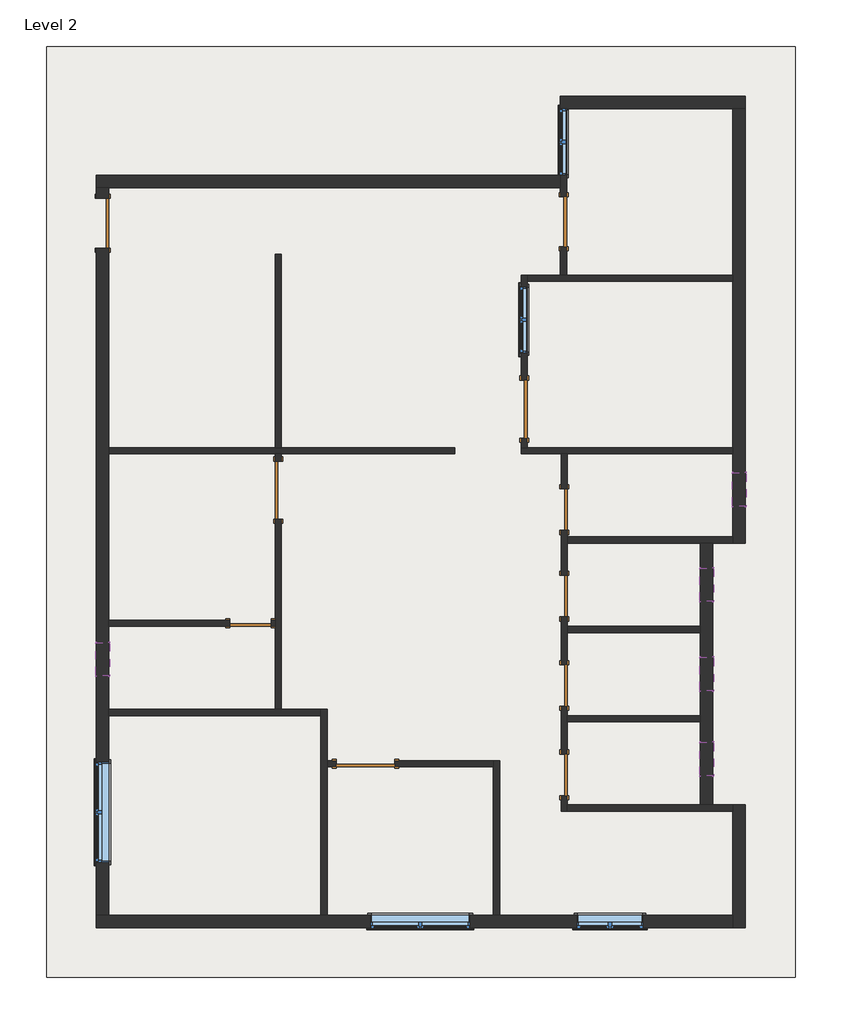
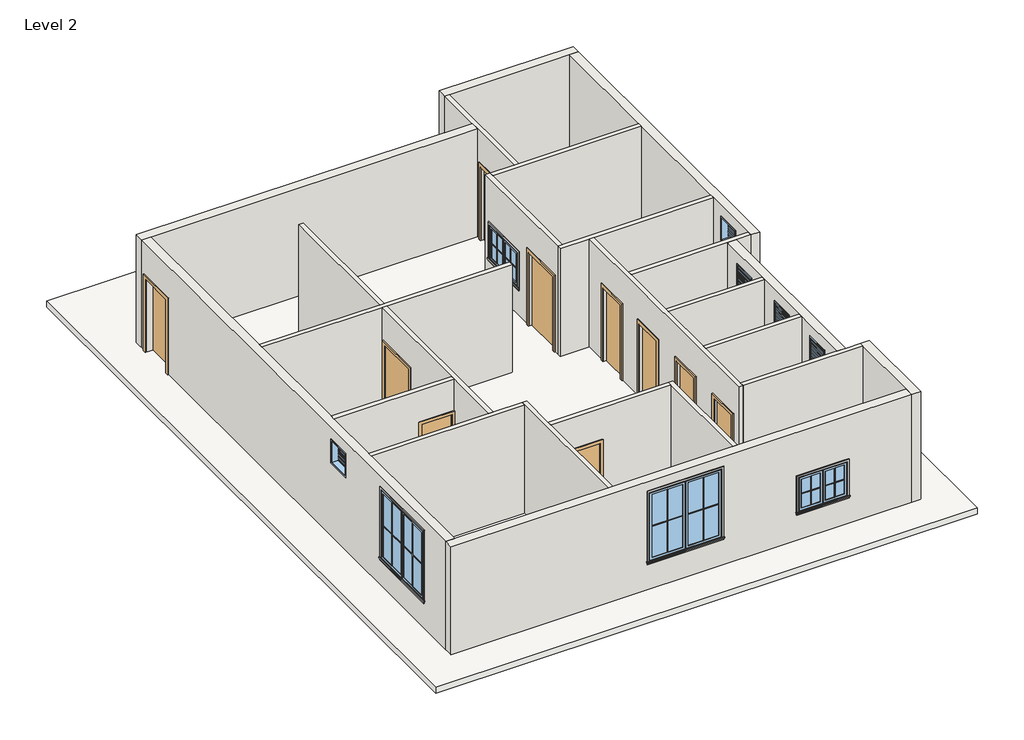
# One storey, incomplete: 23 walls, 20 proxies, 10 doors, 10 windows, 1 roof.
"""IFC4 building model written with IfcOpenShell, lengths in millimetres."""

from ifc_helpers import new_model, si_unit, frame, origin, place, context, project, spatial, polyline, outline, extrude, faceted_brep, transform, mapped, element, save
from components import muntin_pattern_2x2_muntin_pattern_2x2_0a037076, muntin_pattern_2x2_muntin_pattern_2x2_e6f69628, muntin_pattern_2x2_muntin_pattern_2x2_2357e71d, muntin_pattern_2x2_muntin_pattern_2x2_302d8f29, trim_window_exterior_flat_with_sill_b601e94a, trim_window_exterior_flat_with_sill_c4e67c73, trim_window_interior_flat_picture_frame_bfefb25c, trim_window_interior_flat_picture_frame_cf1733af, door_78caadf7, door_214872d5, single_flush_door_3_305aa2a5, single_flush_door_3_a90ba1ad, door_4c162e62, window_casement_double_win_4_c19c33cb, window_casement_double_win_4_2967420f, window_casement_double_win_6_ce442eab, window_f2d8fef0

model = new_model("IFC4")

# Units and contexts
model_context = context("Model", 3, world=origin())
ifc_project = project(units=[si_unit("LENGTHUNIT", "METRE", prefix="MILLI")], contexts=[model_context])

# Site, building, storey
site = spatial("IfcSite", under=ifc_project)
building = spatial("IfcBuilding", under=site)
storey = spatial("IfcBuildingStorey", under=building, Name="Level 2", Elevation=3048.0)

# Proxies
placement = place(None, origin())
muntin_pattern_2x2_muntin_pattern_2x2_shape = muntin_pattern_2x2_muntin_pattern_2x2_0a037076(model_context)
element("IfcBuildingElementProxy", 1, Name="Muntin Pattern_2x2 : Muntin Pattern_2x2", ObjectType="Muntin Pattern_2x2 : Muntin Pattern_2x2", at=placement, inside=storey, context=model_context, shape_type="MappedRepresentation", body=[
    mapped(muntin_pattern_2x2_muntin_pattern_2x2_shape, transform((-7058.058853, -4848.517381, 4032.25), x_axis=(0.0, 1.0, 0.0), y_axis=(-1.0, 0.0, 0.0), z_axis=(0.0, 0.0, 1.0))),
])
element("IfcBuildingElementProxy", 2, Name="Muntin Pattern_2x2 : Muntin Pattern_2x2", ObjectType="Muntin Pattern_2x2 : Muntin Pattern_2x2", at=placement, inside=storey, context=model_context, shape_type="MappedRepresentation", body=[
    mapped(muntin_pattern_2x2_muntin_pattern_2x2_shape, transform((-674.721353, -6497.929881, 4032.25), x_axis=(-1.0, 0.0, 0.0), y_axis=(0.0, -1.0, 0.0), z_axis=(0.0, 0.0, 1.0))),
])
muntin_pattern_2x2_muntin_pattern_2x2_2_shape = muntin_pattern_2x2_muntin_pattern_2x2_e6f69628(model_context)
element("IfcBuildingElementProxy", 3, Name="Muntin Pattern_2x2 : Muntin Pattern_2x2", ObjectType="Muntin Pattern_2x2 : Muntin Pattern_2x2", at=placement, inside=storey, context=model_context, shape_type="MappedRepresentation", body=[
    mapped(muntin_pattern_2x2_muntin_pattern_2x2_2_shape, transform((-7058.058853, -3937.292381, 4032.25), x_axis=(0.0, -1.0, 0.0), y_axis=(1.0, 0.0, 0.0), z_axis=(0.0, 0.0, 1.0))),
])
element("IfcBuildingElementProxy", 4, Name="Muntin Pattern_2x2 : Muntin Pattern_2x2", ObjectType="Muntin Pattern_2x2 : Muntin Pattern_2x2", at=placement, inside=storey, context=model_context, shape_type="MappedRepresentation", body=[
    mapped(muntin_pattern_2x2_muntin_pattern_2x2_2_shape, transform((-1585.946353, -6497.929881, 4032.25), x_axis=(1.0, 0.0, 0.0), y_axis=(0.0, 1.0, 0.0), z_axis=(0.0, 0.0, 1.0))),
])
muntin_pattern_2x2_muntin_pattern_2x2_3_shape = muntin_pattern_2x2_muntin_pattern_2x2_2357e71d(model_context)
element("IfcBuildingElementProxy", 5, Name="Muntin Pattern_2x2 : Muntin Pattern_2x2", ObjectType="Muntin Pattern_2x2 : Muntin Pattern_2x2", at=placement, inside=storey, context=model_context, shape_type="MappedRepresentation", body=[
    mapped(muntin_pattern_2x2_muntin_pattern_2x2_3_shape, transform((2652.678647, -6497.929881, 4032.25), x_axis=(-1.0, 0.0, 0.0), y_axis=(0.0, -1.0, 0.0), z_axis=(0.0, 0.0, 1.0))),
])
element("IfcBuildingElementProxy", 6, Name="Muntin Pattern_2x2 : Muntin Pattern_2x2", ObjectType="Muntin Pattern_2x2 : Muntin Pattern_2x2", at=placement, inside=storey, context=model_context, shape_type="MappedRepresentation", body=[
    mapped(muntin_pattern_2x2_muntin_pattern_2x2_3_shape, transform((727.041147, 4333.582619, 4032.25), x_axis=(0.0, 1.0, 0.0), y_axis=(-1.0, 0.0, 0.0), z_axis=(0.0, 0.0, 1.0))),
])
element("IfcBuildingElementProxy", 7, Name="Muntin Pattern_2x2 : Muntin Pattern_2x2", ObjectType="Muntin Pattern_2x2 : Muntin Pattern_2x2", at=placement, inside=storey, context=model_context, shape_type="MappedRepresentation", body=[
    mapped(muntin_pattern_2x2_muntin_pattern_2x2_3_shape, transform((1450.941147, 7591.132619, 4032.25), x_axis=(0.0, 1.0, 0.0), y_axis=(-1.0, 0.0, 0.0), z_axis=(0.0, 0.0, 1.0))),
])
muntin_pattern_2x2_muntin_pattern_2x2_4_shape = muntin_pattern_2x2_muntin_pattern_2x2_302d8f29(model_context)
element("IfcBuildingElementProxy", 8, Name="Muntin Pattern_2x2 : Muntin Pattern_2x2", ObjectType="Muntin Pattern_2x2 : Muntin Pattern_2x2", at=placement, inside=storey, context=model_context, shape_type="MappedRepresentation", body=[
    mapped(muntin_pattern_2x2_muntin_pattern_2x2_4_shape, transform((2046.253647, -6497.929881, 4032.25), x_axis=(1.0, 0.0, 0.0), y_axis=(0.0, 1.0, 0.0), z_axis=(0.0, 0.0, 1.0))),
])
element("IfcBuildingElementProxy", 9, Name="Muntin Pattern_2x2 : Muntin Pattern_2x2", ObjectType="Muntin Pattern_2x2 : Muntin Pattern_2x2", at=placement, inside=storey, context=model_context, shape_type="MappedRepresentation", body=[
    mapped(muntin_pattern_2x2_muntin_pattern_2x2_4_shape, transform((727.041147, 4940.007619, 4032.25), x_axis=(0.0, -1.0, 0.0), y_axis=(1.0, 0.0, 0.0), z_axis=(0.0, 0.0, 1.0))),
])
element("IfcBuildingElementProxy", 10, Name="Muntin Pattern_2x2 : Muntin Pattern_2x2", ObjectType="Muntin Pattern_2x2 : Muntin Pattern_2x2", at=placement, inside=storey, context=model_context, shape_type="MappedRepresentation", body=[
    mapped(muntin_pattern_2x2_muntin_pattern_2x2_4_shape, transform((1450.941147, 8197.557619, 4032.25), x_axis=(0.0, -1.0, 0.0), y_axis=(1.0, 0.0, 0.0), z_axis=(0.0, 0.0, 1.0))),
])
trim_window_exterior_flat_with_sill_shape = trim_window_exterior_flat_with_sill_b601e94a(model_context)
element("IfcBuildingElementProxy", 11, Name="Trim-Window-Exterior-Flat : with Sill", ObjectType="Trim-Window-Exterior-Flat : with Sill", at=placement, inside=storey, context=model_context, shape_type="MappedRepresentation", body=[
    mapped(trim_window_exterior_flat_with_sill_shape, transform((-7067.583853, -4392.904881, 5791.2), x_axis=(0.0, -1.0, 0.0), y_axis=(0.0, 0.0, 1.0), z_axis=(-1.0, 0.0, 0.0))),
])
element("IfcBuildingElementProxy", 12, Name="Trim-Window-Exterior-Flat : with Sill", ObjectType="Trim-Window-Exterior-Flat : with Sill", at=placement, inside=storey, context=model_context, shape_type="MappedRepresentation", body=[
    mapped(trim_window_exterior_flat_with_sill_shape, transform((-1130.333853, -6507.454881, 5791.2), x_axis=(1.0, 0.0, 0.0), y_axis=(0.0, 0.0, 1.0), z_axis=(0.0, -1.0, 0.0))),
])
trim_window_exterior_flat_with_sill_2_shape = trim_window_exterior_flat_with_sill_c4e67c73(model_context)
element("IfcBuildingElementProxy", 13, Name="Trim-Window-Exterior-Flat : with Sill", ObjectType="Trim-Window-Exterior-Flat : with Sill", at=placement, inside=storey, context=model_context, shape_type="MappedRepresentation", body=[
    mapped(trim_window_exterior_flat_with_sill_2_shape, transform((2349.466147, -6507.454881, 4876.8), x_axis=(1.0, 0.0, 0.0), y_axis=(0.0, 0.0, 1.0), z_axis=(0.0, -1.0, 0.0))),
])
element("IfcBuildingElementProxy", 14, Name="Trim-Window-Exterior-Flat : with Sill", ObjectType="Trim-Window-Exterior-Flat : with Sill", at=placement, inside=storey, context=model_context, shape_type="MappedRepresentation", body=[
    mapped(trim_window_exterior_flat_with_sill_2_shape, transform((717.516147, 4636.795119, 4876.8), x_axis=(0.0, -1.0, 0.0), y_axis=(0.0, 0.0, 1.0), z_axis=(-1.0, 0.0, 0.0))),
])
element("IfcBuildingElementProxy", 15, Name="Trim-Window-Exterior-Flat : with Sill", ObjectType="Trim-Window-Exterior-Flat : with Sill", at=placement, inside=storey, context=model_context, shape_type="MappedRepresentation", body=[
    mapped(trim_window_exterior_flat_with_sill_2_shape, transform((1441.416147, 7894.345119, 4876.8), x_axis=(0.0, -1.0, 0.0), y_axis=(0.0, 0.0, 1.0), z_axis=(-1.0, 0.0, 0.0))),
])
trim_window_interior_flat_picture_frame_shape = trim_window_interior_flat_picture_frame_bfefb25c(model_context)
element("IfcBuildingElementProxy", 16, Name="Trim-Window-Interior-Flat : Picture Frame", ObjectType="Trim-Window-Interior-Flat : Picture Frame", at=placement, inside=storey, context=model_context, shape_type="MappedRepresentation", body=[
    mapped(trim_window_interior_flat_picture_frame_shape, transform((-6838.983853, -4392.904881, 5791.2), x_axis=(0.0, 1.0, 0.0), y_axis=(0.0, 0.0, 1.0), z_axis=(1.0, 0.0, 0.0))),
])
element("IfcBuildingElementProxy", 17, Name="Trim-Window-Interior-Flat : Picture Frame", ObjectType="Trim-Window-Interior-Flat : Picture Frame", at=placement, inside=storey, context=model_context, shape_type="MappedRepresentation", body=[
    mapped(trim_window_interior_flat_picture_frame_shape, transform((-1130.333853, -6278.854881, 5791.2), x_axis=(-1.0, 0.0, 0.0), y_axis=(0.0, 0.0, 1.0), z_axis=(0.0, 1.0, 0.0))),
])
trim_window_interior_flat_picture_frame_2_shape = trim_window_interior_flat_picture_frame_cf1733af(model_context)
element("IfcBuildingElementProxy", 18, Name="Trim-Window-Interior-Flat : Picture Frame", ObjectType="Trim-Window-Interior-Flat : Picture Frame", at=placement, inside=storey, context=model_context, shape_type="MappedRepresentation", body=[
    mapped(trim_window_interior_flat_picture_frame_2_shape, transform((2349.466147, -6278.854881, 4876.8), x_axis=(-1.0, 0.0, 0.0), y_axis=(0.0, 0.0, 1.0), z_axis=(0.0, 1.0, 0.0))),
])
element("IfcBuildingElementProxy", 19, Name="Trim-Window-Interior-Flat : Picture Frame", ObjectType="Trim-Window-Interior-Flat : Picture Frame", at=placement, inside=storey, context=model_context, shape_type="MappedRepresentation", body=[
    mapped(trim_window_interior_flat_picture_frame_2_shape, transform((831.816147, 4636.795119, 4876.8), x_axis=(0.0, 1.0, 0.0), y_axis=(0.0, 0.0, 1.0), z_axis=(1.0, 0.0, 0.0))),
])
element("IfcBuildingElementProxy", 20, Name="Trim-Window-Interior-Flat : Picture Frame", ObjectType="Trim-Window-Interior-Flat : Picture Frame", at=placement, inside=storey, context=model_context, shape_type="MappedRepresentation", body=[
    mapped(trim_window_interior_flat_picture_frame_2_shape, transform((1555.716147, 7894.345119, 4876.8), x_axis=(0.0, 1.0, 0.0), y_axis=(0.0, 0.0, 1.0), z_axis=(1.0, 0.0, 0.0))),
])

# Doors
door_shape = door_78caadf7(model_context)
element("IfcDoor", 21, ObjectType="Single-Flush : 2'6\"", at=placement, inside=storey, context=model_context, shape_type="MappedRepresentation", body=[
    mapped(door_shape, transform((-4241.833853, -925.804881, 3048.0), x_axis=(1.0, 0.0, 0.0), y_axis=(0.0, 1.0, 0.0), z_axis=(0.0, 0.0, 1.0))),
])
door_2_shape = door_214872d5(model_context)
element("IfcDoor", 22, ObjectType="Single-Flush : 2'6\"", at=placement, inside=storey, context=model_context, shape_type="MappedRepresentation", body=[
    mapped(door_2_shape, transform((1511.266147, 1156.995119, 3048.0), x_axis=(0.0, -1.0, 0.0), y_axis=(1.0, 0.0, 0.0), z_axis=(0.0, 0.0, 1.0))),
])
element("IfcDoor", 23, ObjectType="Single-Flush : 2'6\"", at=placement, inside=storey, context=model_context, shape_type="MappedRepresentation", body=[
    mapped(door_2_shape, transform((1511.266147, -430.504881, 3048.0), x_axis=(0.0, -1.0, 0.0), y_axis=(1.0, 0.0, 0.0), z_axis=(0.0, 0.0, 1.0))),
])
element("IfcDoor", 24, ObjectType="Single-Flush : 2'6\"", at=placement, inside=storey, context=model_context, shape_type="MappedRepresentation", body=[
    mapped(door_2_shape, transform((1511.266147, -2068.804881, 3048.0), x_axis=(0.0, -1.0, 0.0), y_axis=(1.0, 0.0, 0.0), z_axis=(0.0, 0.0, 1.0))),
])
element("IfcDoor", 25, ObjectType="Single-Flush : 2'6\"", at=placement, inside=storey, context=model_context, shape_type="MappedRepresentation", body=[
    mapped(door_2_shape, transform((1511.266147, -3707.104881, 3048.0), x_axis=(0.0, -1.0, 0.0), y_axis=(1.0, 0.0, 0.0), z_axis=(0.0, 0.0, 1.0))),
])
single_flush_door_3_shape = single_flush_door_3_305aa2a5(model_context)
element("IfcDoor", 26, ObjectType="Single-Flush : DOOR 3'", at=placement, inside=storey, context=model_context, shape_type="MappedRepresentation", body=[
    mapped(single_flush_door_3_shape, transform((1498.566147, 6433.845119, 3048.0), x_axis=(0.0, 1.0, 0.0), y_axis=(-1.0, 0.0, 0.0), z_axis=(0.0, 0.0, 1.0))),
])
single_flush_door_3_2_shape = single_flush_door_3_a90ba1ad(model_context)
element("IfcDoor", 27, ObjectType="Single-Flush : DOOR 3'", at=placement, inside=storey, context=model_context, shape_type="MappedRepresentation", body=[
    mapped(single_flush_door_3_2_shape, transform((-6953.283853, 6408.445119, 3048.0), x_axis=(0.0, 1.0, 0.0), y_axis=(-1.0, 0.0, 0.0), z_axis=(0.0, 0.0, 1.0))),
])
door_3_shape = door_4c162e62(model_context)
element("IfcDoor", 28, ObjectType="Single-Flush : DOOR 3'6\"", at=placement, inside=storey, context=model_context, shape_type="MappedRepresentation", body=[
    mapped(door_3_shape, transform((-3733.833853, 1512.595119, 3048.0), x_axis=(0.0, 1.0, 0.0), y_axis=(-1.0, 0.0, 0.0), z_axis=(0.0, 0.0, 1.0))),
])
element("IfcDoor", 29, ObjectType="Single-Flush : DOOR 3'6\"", at=placement, inside=storey, context=model_context, shape_type="MappedRepresentation", body=[
    mapped(door_3_shape, transform((774.666147, 2998.495119, 3048.0), x_axis=(0.0, -1.0, 0.0), y_axis=(1.0, 0.0, 0.0), z_axis=(0.0, 0.0, 1.0))),
])
element("IfcDoor", 30, ObjectType="Single-Flush : DOOR 3'6\"", at=placement, inside=storey, context=model_context, shape_type="MappedRepresentation", body=[
    mapped(door_3_shape, transform((-2133.633853, -3503.904881, 3048.0), x_axis=(-1.0, 0.0, 0.0), y_axis=(0.0, -1.0, 0.0), z_axis=(0.0, 0.0, 1.0))),
])

# Roof
element("IfcRoof", 31, ObjectType="Generic - 12\"", at=placement, inside=storey, context=model_context, shape_type="SweptSolid", body=[
    extrude(outline(polyline([(-7981.983853, 9646.945119), (5746.716147, 9646.945119), (5746.716147, -7421.854881), (-7981.983853, -7421.854881), (-7981.983853, 9646.945119)])), frame((0.0, 0.0, 3048.0), z_axis=(0.0, 0.0, 1.0), x_axis=(1.0, 0.0, 0.0)), (0.0, 0.0, 1.0), 152.4),
])

# Walls
element("IfcWall", 32, ObjectType="WALL 4.5\"", at=placement, inside=storey, context=model_context, shape_type="Brep", body=[
    faceted_brep([(-6838.983853, 2179.345119, 3048.0), (-3790.983853, 2179.345119, 3048.0), (-3676.683853, 2179.345119, 3048.0), (-501.683853, 2179.345119, 3048.0), (-501.683853, 2179.345119, 6096.0), (-3676.683853, 2179.345119, 6096.0), (-3790.983853, 2179.345119, 6096.0), (-6838.983853, 2179.345119, 6096.0), (-6838.983853, 2293.645119, 3048.0), (-6838.983853, 2293.645119, 6096.0), (-3790.983853, 2293.645119, 6096.0), (-3676.683853, 2293.645119, 6096.0), (-501.683853, 2293.645119, 6096.0), (-501.683853, 2293.645119, 3048.0), (-3676.683853, 2293.645119, 3048.0), (-3790.983853, 2293.645119, 3048.0)], [[[0, 1, 2, 3, 4, 5, 6, 7]], [[8, 9, 10, 11, 12, 13, 14, 15]], [[3, 2, 1, 0, 8, 15, 14, 13]], [[4, 3, 13, 12]], [[0, 7, 9, 8]], [[7, 6, 5, 4, 12, 11, 10, 9]]]),
])
element("IfcWall", 33, ObjectType="WALL 4.5\"", at=placement, inside=storey, context=model_context, shape_type="Brep", body=[
    faceted_brep([(-2838.483853, -6278.854881, 3048.0), (-2838.483853, -3561.054881, 3048.0), (-2838.483853, -3446.754881, 3048.0), (-2838.483853, -2506.954881, 3048.0), (-2838.483853, -2506.954881, 6096.0), (-2838.483853, -3446.754881, 6096.0), (-2838.483853, -3561.054881, 6096.0), (-2838.483853, -6278.854881, 6096.0), (-2952.783853, -6278.854881, 3048.0), (-2952.783853, -6278.854881, 6096.0), (-2952.783853, -2621.254881, 6096.0), (-2952.783853, -2506.954881, 6096.0), (-2952.783853, -2506.954881, 3048.0), (-2952.783853, -2621.254881, 3048.0)], [[[0, 1, 2, 3, 4, 5, 6, 7]], [[8, 9, 10, 11, 12, 13]], [[3, 2, 1, 0, 8, 13, 12]], [[0, 7, 9, 8]], [[4, 3, 12, 11]], [[7, 6, 5, 4, 11, 10, 9]]]),
])
element("IfcWall", 34, ObjectType="WALL 4.5\"", at=placement, inside=storey, context=model_context, shape_type="Brep", body=[
    faceted_brep([(-2952.783853, -2506.954881, 3048.0), (-3676.683853, -2506.954881, 3048.0), (-3790.983853, -2506.954881, 3048.0), (-6838.983853, -2506.954881, 3048.0), (-6838.983853, -2506.954881, 6096.0), (-3790.983853, -2506.954881, 6096.0), (-3676.683853, -2506.954881, 6096.0), (-2952.783853, -2506.954881, 6096.0), (-2952.783853, -2621.254881, 3048.0), (-2952.783853, -2621.254881, 6096.0), (-6838.983853, -2621.254881, 6096.0), (-6838.983853, -2621.254881, 3048.0)], [[[0, 1, 2, 3, 4, 5, 6, 7]], [[8, 9, 10, 11]], [[3, 2, 1, 0, 8, 11]], [[0, 7, 9, 8]], [[4, 3, 11, 10]], [[7, 6, 5, 4, 10, 9]]]),
])
element("IfcWall", 35, ObjectType="WALL 4.5\"", at=placement, inside=storey, context=model_context, shape_type="SweptSolid", body=[
    extrude(outline(polyline([(5181.6, -3860.833853), (3048.0, -3860.833853), (3048.0, -3790.983853), (6096.0, -3790.983853), (6096.0, -6838.983853), (3048.0, -6838.983853), (3048.0, -4622.833853), (5181.6, -4622.833853), (5181.6, -3860.833853)])), frame((0.0, -982.954881, 0.0), z_axis=(0.0, 1.0, 0.0), x_axis=(0.0, 0.0, 1.0)), (0.0, 0.0, 1.0), 114.3),
])
element("IfcWall", 36, ObjectType="WALL 4.5\"", at=placement, inside=storey, context=model_context, shape_type="Brep", body=[
    faceted_brep([(-3676.683853, 5836.945119, 3048.0), (-3676.683853, 5836.945119, 6096.0), (-3676.683853, 2293.645119, 6096.0), (-3676.683853, 2293.645119, 3048.0), (-3790.983853, 5836.945119, 6096.0), (-3790.983853, 5836.945119, 3048.0), (-3790.983853, 2293.645119, 3048.0), (-3790.983853, 2293.645119, 6096.0)], [[[0, 1, 2, 3]], [[4, 5, 6, 7]], [[5, 0, 3, 6]], [[1, 0, 5, 4]], [[3, 2, 7, 6]], [[1, 4, 7, 2]]]),
    faceted_brep([(-3676.683853, -2506.954881, 6096.0), (-3676.683853, -2506.954881, 3048.0), (-3676.683853, 979.195119, 3048.0), (-3676.683853, 979.195119, 5181.6), (-3676.683853, 2045.995119, 5181.6), (-3676.683853, 2045.995119, 3048.0), (-3676.683853, 2179.345119, 3048.0), (-3676.683853, 2179.345119, 6096.0), (-3790.983853, -2506.954881, 3048.0), (-3790.983853, -2506.954881, 6096.0), (-3790.983853, -982.954881, 6096.0), (-3790.983853, -868.654881, 6096.0), (-3790.983853, 2179.345119, 6096.0), (-3790.983853, 2179.345119, 3048.0), (-3790.983853, 2045.995119, 3048.0), (-3790.983853, 2045.995119, 5181.6), (-3790.983853, 979.195119, 5181.6), (-3790.983853, 979.195119, 3048.0), (-3790.983853, -868.654881, 3048.0), (-3790.983853, -982.954881, 3048.0)], [[[0, 1, 2, 3, 4, 5, 6, 7]], [[8, 9, 10, 11, 12, 13, 14, 15, 16, 17, 18, 19]], [[1, 8, 19, 18, 17, 2]], [[5, 14, 13, 6]], [[1, 0, 9, 8]], [[7, 6, 13, 12]], [[15, 14, 5, 4]], [[16, 15, 4, 3]], [[17, 16, 3, 2]], [[9, 0, 7, 12, 11, 10]]]),
])
element("IfcWall", 37, ObjectType="WALL 4.5\"", at=placement, inside=storey, context=model_context, shape_type="Brep", body=[
    faceted_brep([(4603.716147, 2293.645119, 3048.0), (831.816147, 2293.645119, 3048.0), (717.516147, 2293.645119, 3048.0), (717.516147, 2293.645119, 6096.0), (831.816147, 2293.645119, 6096.0), (4603.716147, 2293.645119, 6096.0), (4603.716147, 2179.345119, 3048.0), (4603.716147, 2179.345119, 6096.0), (1568.416147, 2179.345119, 6096.0), (1454.116147, 2179.345119, 6096.0), (717.516147, 2179.345119, 6096.0), (717.516147, 2179.345119, 3048.0), (1454.116147, 2179.345119, 3048.0), (1568.416147, 2179.345119, 3048.0)], [[[0, 1, 2, 3, 4, 5]], [[6, 7, 8, 9, 10, 11, 12, 13]], [[2, 1, 0, 6, 13, 12, 11]], [[0, 5, 7, 6]], [[3, 2, 11, 10]], [[5, 4, 3, 10, 9, 8, 7]]]),
])
element("IfcWall", 38, ObjectType="WALL 4.5\"", at=placement, inside=storey, context=model_context, shape_type="Brep", body=[
    faceted_brep([(831.816147, 2293.645119, 3048.0), (831.816147, 2465.095119, 3048.0), (831.816147, 2465.095119, 5181.6), (831.816147, 3531.895119, 5181.6), (831.816147, 3531.895119, 3048.0), (831.816147, 5341.645119, 3048.0), (831.816147, 5455.945119, 3048.0), (831.816147, 5455.945119, 6096.0), (831.816147, 5341.645119, 6096.0), (831.816147, 2293.645119, 6096.0), (831.816147, 5246.395119, 4876.8), (831.816147, 5246.395119, 3962.4), (831.816147, 4027.195119, 3962.4), (831.816147, 4027.195119, 4876.8), (717.516147, 2465.095119, 5181.6), (717.516147, 2465.095119, 3048.0), (717.516147, 2293.645119, 3048.0), (717.516147, 2293.645119, 6096.0), (717.516147, 5455.945119, 6096.0), (717.516147, 5455.945119, 3048.0), (717.516147, 3531.895119, 3048.0), (717.516147, 3531.895119, 5181.6), (717.516147, 5246.395119, 4876.8), (717.516147, 4027.195119, 4876.8), (717.516147, 4027.195119, 3962.4), (717.516147, 5246.395119, 3962.4)], [[[0, 1, 2, 3, 4, 5, 6, 7, 8, 9], [10, 11, 12, 13]], [[14, 15, 16, 17, 18, 19, 20, 21], [22, 23, 24, 25]], [[20, 19, 6, 5, 4]], [[16, 15, 1, 0]], [[0, 9, 17, 16]], [[7, 6, 19, 18]], [[11, 10, 22, 25]], [[12, 11, 25, 24]], [[13, 12, 24, 23]], [[10, 13, 23, 22]], [[2, 1, 15, 14]], [[3, 2, 14, 21]], [[4, 3, 21, 20]], [[9, 8, 7, 18, 17]]]),
])
element("IfcWall", 39, ObjectType="WALL 4.5\"", at=placement, inside=storey, context=model_context, shape_type="Brep", body=[
    faceted_brep([(831.816147, 5341.645119, 3048.0), (4603.716147, 5341.645119, 3048.0), (4603.716147, 5341.645119, 6096.0), (831.816147, 5341.645119, 6096.0), (831.816147, 5455.945119, 3048.0), (831.816147, 5455.945119, 6096.0), (1441.416147, 5455.945119, 6096.0), (1555.716147, 5455.945119, 6096.0), (4603.716147, 5455.945119, 6096.0), (4603.716147, 5455.945119, 3048.0), (1555.716147, 5455.945119, 3048.0), (1441.416147, 5455.945119, 3048.0)], [[[0, 1, 2, 3]], [[4, 5, 6, 7, 8, 9, 10, 11]], [[1, 0, 4, 11, 10, 9]], [[0, 3, 5, 4]], [[2, 1, 9, 8]], [[3, 2, 8, 7, 6, 5]]]),
])
element("IfcWall", 40, ObjectType="WALL 4.5\"", at=placement, inside=storey, context=model_context, shape_type="Brep", body=[
    faceted_brep([(1555.716147, 6891.045119, 5181.6), (1555.716147, 6891.045119, 3048.0), (1555.716147, 8503.945119, 3048.0), (1555.716147, 8503.945119, 3962.4), (1555.716147, 7284.745119, 3962.4), (1555.716147, 7284.745119, 4876.8), (1555.716147, 8503.945119, 4876.8), (1555.716147, 8503.945119, 6096.0), (1555.716147, 5455.945119, 6096.0), (1555.716147, 5455.945119, 3048.0), (1555.716147, 5976.645119, 3048.0), (1555.716147, 5976.645119, 5181.6), (1441.416147, 8503.945119, 3048.0), (1441.416147, 7284.745119, 3048.0), (1441.416147, 7056.145119, 3048.0), (1441.416147, 6891.045119, 3048.0), (1441.416147, 6891.045119, 5181.6), (1441.416147, 5976.645119, 5181.6), (1441.416147, 5976.645119, 3048.0), (1441.416147, 5455.945119, 3048.0), (1441.416147, 5455.945119, 6096.0), (1441.416147, 7056.145119, 6096.0), (1441.416147, 7284.745119, 6096.0), (1441.416147, 8503.945119, 6096.0), (1441.416147, 8503.945119, 4876.8), (1441.416147, 7284.745119, 4876.8), (1441.416147, 7284.745119, 3962.4), (1441.416147, 8503.945119, 3962.4)], [[[0, 1, 2, 3, 4, 5, 6, 7, 8, 9, 10, 11]], [[12, 13, 14, 15, 16, 17, 18, 19, 20, 21, 22, 23, 24, 25, 26, 27]], [[10, 9, 19, 18]], [[2, 1, 15, 14, 13, 12]], [[24, 23, 7, 6]], [[12, 27, 3, 2]], [[9, 8, 20, 19]], [[4, 3, 27, 26]], [[5, 4, 26, 25]], [[6, 5, 25, 24]], [[16, 15, 1, 0]], [[17, 16, 0, 11]], [[18, 17, 11, 10]], [[8, 7, 23, 22, 21, 20]]]),
])
element("IfcWall", 41, ObjectType="WALL 4.5\"", at=placement, inside=storey, context=model_context, shape_type="Brep", body=[
    faceted_brep([(4603.716147, 655.345119, 3048.0), (1568.416147, 655.345119, 3048.0), (1568.416147, 655.345119, 6096.0), (4603.716147, 655.345119, 6096.0), (4603.716147, 541.045119, 3048.0), (4603.716147, 541.045119, 6096.0), (4235.416147, 541.045119, 6096.0), (4006.816147, 541.045119, 6096.0), (1568.416147, 541.045119, 6096.0), (1568.416147, 541.045119, 3048.0), (4006.816147, 541.045119, 3048.0), (4235.416147, 541.045119, 3048.0)], [[[0, 1, 2, 3]], [[4, 5, 6, 7, 8, 9, 10, 11]], [[1, 0, 4, 11, 10, 9]], [[0, 3, 5, 4]], [[2, 1, 9, 8]], [[3, 2, 8, 7, 6, 5]]]),
])
element("IfcWall", 42, ObjectType="WALL 4.5\"", at=placement, inside=storey, context=model_context, shape_type="Brep", body=[
    faceted_brep([(1454.116147, -4088.104881, 5181.6), (1454.116147, -4088.104881, 3048.0), (1454.116147, -4373.854881, 3048.0), (1454.116147, -4373.854881, 6096.0), (1454.116147, 2179.345119, 6096.0), (1454.116147, 2179.345119, 3048.0), (1454.116147, 1537.995119, 3048.0), (1454.116147, 1537.995119, 5181.6), (1454.116147, 775.995119, 5181.6), (1454.116147, 775.995119, 3048.0), (1454.116147, -49.504881, 3048.0), (1454.116147, -49.504881, 5181.6), (1454.116147, -811.504881, 5181.6), (1454.116147, -811.504881, 3048.0), (1454.116147, -1687.804881, 3048.0), (1454.116147, -1687.804881, 5181.6), (1454.116147, -2449.804881, 5181.6), (1454.116147, -2449.804881, 3048.0), (1454.116147, -3326.104881, 3048.0), (1454.116147, -3326.104881, 5181.6), (1568.416147, -4373.854881, 3048.0), (1568.416147, -4259.554881, 3048.0), (1568.416147, -4088.104881, 3048.0), (1568.416147, -4088.104881, 5181.6), (1568.416147, -3326.104881, 5181.6), (1568.416147, -3326.104881, 3048.0), (1568.416147, -2735.554881, 3048.0), (1568.416147, -2621.254881, 3048.0), (1568.416147, -2449.804881, 3048.0), (1568.416147, -2449.804881, 5181.6), (1568.416147, -1687.804881, 5181.6), (1568.416147, -1687.804881, 3048.0), (1568.416147, -1097.254881, 3048.0), (1568.416147, -982.954881, 3048.0), (1568.416147, -811.504881, 3048.0), (1568.416147, -811.504881, 5181.6), (1568.416147, -49.504881, 5181.6), (1568.416147, -49.504881, 3048.0), (1568.416147, 541.045119, 3048.0), (1568.416147, 655.345119, 3048.0), (1568.416147, 775.995119, 3048.0), (1568.416147, 775.995119, 5181.6), (1568.416147, 1537.995119, 5181.6), (1568.416147, 1537.995119, 3048.0), (1568.416147, 2179.345119, 3048.0), (1568.416147, 2179.345119, 6096.0), (1568.416147, 655.345119, 6096.0), (1568.416147, 541.045119, 6096.0), (1568.416147, -982.954881, 6096.0), (1568.416147, -1097.254881, 6096.0), (1568.416147, -2621.254881, 6096.0), (1568.416147, -2735.554881, 6096.0), (1568.416147, -4259.554881, 6096.0), (1568.416147, -4373.854881, 6096.0)], [[[0, 1, 2, 3, 4, 5, 6, 7, 8, 9, 10, 11, 12, 13, 14, 15, 16, 17, 18, 19]], [[20, 21, 22, 23, 24, 25, 26, 27, 28, 29, 30, 31, 32, 33, 34, 35, 36, 37, 38, 39, 40, 41, 42, 43, 44, 45, 46, 47, 48, 49, 50, 51, 52, 53]], [[6, 5, 44, 43]], [[10, 9, 40, 39, 38, 37]], [[14, 13, 34, 33, 32, 31]], [[18, 17, 28, 27, 26, 25]], [[2, 1, 22, 21, 20]], [[5, 4, 45, 44]], [[3, 2, 20, 53]], [[41, 40, 9, 8]], [[42, 41, 8, 7]], [[43, 42, 7, 6]], [[35, 34, 13, 12]], [[36, 35, 12, 11]], [[37, 36, 11, 10]], [[29, 28, 17, 16]], [[30, 29, 16, 15]], [[31, 30, 15, 14]], [[23, 22, 1, 0]], [[24, 23, 0, 19]], [[25, 24, 19, 18]], [[4, 3, 53, 52, 51, 50, 49, 48, 47, 46, 45]]]),
])
element("IfcWall", 43, ObjectType="WALL 4.5\"", at=placement, inside=storey, context=model_context, shape_type="Brep", body=[
    faceted_brep([(1568.416147, -4373.854881, 3048.0), (4603.716147, -4373.854881, 3048.0), (4603.716147, -4373.854881, 6096.0), (1568.416147, -4373.854881, 6096.0), (1568.416147, -4259.554881, 3048.0), (1568.416147, -4259.554881, 6096.0), (4006.816147, -4259.554881, 6096.0), (4235.416147, -4259.554881, 6096.0), (4603.716147, -4259.554881, 6096.0), (4603.716147, -4259.554881, 3048.0), (4235.416147, -4259.554881, 3048.0), (4006.816147, -4259.554881, 3048.0)], [[[0, 1, 2, 3]], [[4, 5, 6, 7, 8, 9, 10, 11]], [[1, 0, 4, 11, 10, 9]], [[0, 3, 5, 4]], [[2, 1, 9, 8]], [[3, 2, 8, 7, 6, 5]]]),
])
element("IfcWall", 44, ObjectType="WALL 4.5\"", at=placement, inside=storey, context=model_context, shape_type="SweptSolid", body=[
    extrude(outline(polyline([(4006.816147, -2735.554881), (1568.416147, -2735.554881), (1568.416147, -2621.254881), (4006.816147, -2621.254881), (4006.816147, -2735.554881)])), frame((0.0, 0.0, 3048.0), z_axis=(0.0, 0.0, 1.0), x_axis=(1.0, 0.0, 0.0)), (0.0, 0.0, 1.0), 3048.0),
])
element("IfcWall", 45, ObjectType="WALL 4.5\"", at=placement, inside=storey, context=model_context, shape_type="SweptSolid", body=[
    extrude(outline(polyline([(4006.816147, -1097.254881), (1568.416147, -1097.254881), (1568.416147, -982.954881), (4006.816147, -982.954881), (4006.816147, -1097.254881)])), frame((0.0, 0.0, 3048.0), z_axis=(0.0, 0.0, 1.0), x_axis=(1.0, 0.0, 0.0)), (0.0, 0.0, 1.0), 3048.0),
])
element("IfcWall", 46, ObjectType="WALL 4.5\"", at=placement, inside=storey, context=model_context, shape_type="Brep", body=[
    faceted_brep([(323.816147, -6278.854881, 3048.0), (323.816147, -3446.754881, 3048.0), (323.816147, -3446.754881, 6096.0), (323.816147, -6278.854881, 6096.0), (209.516147, -6278.854881, 3048.0), (209.516147, -6278.854881, 6096.0), (209.516147, -3561.054881, 6096.0), (209.516147, -3446.754881, 6096.0), (209.516147, -3446.754881, 3048.0), (209.516147, -3561.054881, 3048.0)], [[[0, 1, 2, 3]], [[4, 5, 6, 7, 8, 9]], [[1, 0, 4, 9, 8]], [[0, 3, 5, 4]], [[2, 1, 8, 7]], [[3, 2, 7, 6, 5]]]),
])
element("IfcWall", 47, ObjectType="WALL 4.5\"", at=placement, inside=storey, context=model_context, shape_type="SweptSolid", body=[
    extrude(outline(polyline([(3048.0, -2838.483853), (3048.0, -2667.033853), (5181.6, -2667.033853), (5181.6, -1600.233853), (3048.0, -1600.233853), (3048.0, 209.516147), (6096.0, 209.516147), (6096.0, -2838.483853), (3048.0, -2838.483853)])), frame((0.0, -3561.054881, 0.0), z_axis=(0.0, 1.0, 0.0), x_axis=(0.0, 0.0, 1.0)), (0.0, 0.0, 1.0), 114.3),
])
element("IfcWall", 48, ObjectType="WALL 9\"", at=placement, inside=storey, context=model_context, shape_type="Brep", body=[
    faceted_brep([(-7067.583853, 7056.145119, 3048.0), (-6838.983853, 7056.145119, 3048.0), (1441.416147, 7056.145119, 3048.0), (1441.416147, 7056.145119, 6096.0), (-6838.983853, 7056.145119, 6096.0), (-7067.583853, 7056.145119, 6096.0), (-7067.583853, 7284.745119, 3048.0), (-7067.583853, 7284.745119, 6096.0), (1441.416147, 7284.745119, 6096.0), (1441.416147, 7284.745119, 3048.0)], [[[0, 1, 2, 3, 4, 5]], [[6, 7, 8, 9]], [[2, 1, 0, 6, 9]], [[0, 5, 7, 6]], [[3, 2, 9, 8]], [[5, 4, 3, 8, 7]]]),
])
element("IfcWall", 49, ObjectType="WALL 9\"", at=placement, inside=storey, context=model_context, shape_type="Brep", body=[
    faceted_brep([(1441.416147, 8503.945119, 3048.0), (1555.716147, 8503.945119, 3048.0), (4603.716147, 8503.945119, 3048.0), (4832.316147, 8503.945119, 3048.0), (4832.316147, 8503.945119, 6096.0), (4603.716147, 8503.945119, 6096.0), (1555.716147, 8503.945119, 6096.0), (1441.416147, 8503.945119, 6096.0), (1441.416147, 8503.945119, 4876.8), (1441.416147, 8503.945119, 3962.4), (1441.416147, 8732.545119, 3048.0), (1441.416147, 8732.545119, 6096.0), (4832.316147, 8732.545119, 6096.0), (4832.316147, 8732.545119, 3048.0)], [[[0, 1, 2, 3, 4, 5, 6, 7, 8, 9]], [[10, 11, 12, 13]], [[3, 2, 1, 0, 10, 13]], [[4, 3, 13, 12]], [[0, 9, 8, 7, 11, 10]], [[7, 6, 5, 4, 12, 11]]]),
])
element("IfcWall", 50, ObjectType="WALL 9\"", at=placement, inside=storey, context=model_context, shape_type="Brep", body=[
    faceted_brep([(4603.716147, 8503.945119, 3048.0), (4603.716147, 5455.945119, 3048.0), (4603.716147, 5341.645119, 3048.0), (4603.716147, 2293.645119, 3048.0), (4603.716147, 2179.345119, 3048.0), (4603.716147, 655.345119, 3048.0), (4603.716147, 541.045119, 3048.0), (4603.716147, 541.045119, 6096.0), (4603.716147, 655.345119, 6096.0), (4603.716147, 2179.345119, 6096.0), (4603.716147, 2293.645119, 6096.0), (4603.716147, 5341.645119, 6096.0), (4603.716147, 5455.945119, 6096.0), (4603.716147, 8503.945119, 6096.0), (4603.716147, 1830.095119, 5791.2), (4603.716147, 1220.495119, 5791.2), (4603.716147, 1220.495119, 5181.6), (4603.716147, 1830.095119, 5181.6), (4832.316147, 8503.945119, 3048.0), (4832.316147, 8503.945119, 6096.0), (4832.316147, 541.045119, 6096.0), (4832.316147, 541.045119, 3048.0), (4832.316147, 1830.095119, 5791.2), (4832.316147, 1830.095119, 5181.6), (4832.316147, 1220.495119, 5181.6), (4832.316147, 1220.495119, 5791.2)], [[[0, 1, 2, 3, 4, 5, 6, 7, 8, 9, 10, 11, 12, 13], [14, 15, 16, 17]], [[18, 19, 20, 21], [22, 23, 24, 25]], [[6, 5, 4, 3, 2, 1, 0, 18, 21]], [[0, 13, 19, 18]], [[7, 6, 21, 20]], [[23, 22, 14, 17]], [[24, 23, 17, 16]], [[25, 24, 16, 15]], [[22, 25, 15, 14]], [[13, 12, 11, 10, 9, 8, 7, 20, 19]]]),
])
element("IfcWall", 51, ObjectType="WALL 9\"", at=placement, inside=storey, context=model_context, shape_type="Brep", body=[
    faceted_brep([(4006.816147, 541.045119, 3048.0), (4006.816147, -982.954881, 3048.0), (4006.816147, -1097.254881, 3048.0), (4006.816147, -2621.254881, 3048.0), (4006.816147, -2735.554881, 3048.0), (4006.816147, -4259.554881, 3048.0), (4006.816147, -4259.554881, 6096.0), (4006.816147, -2735.554881, 6096.0), (4006.816147, -2621.254881, 6096.0), (4006.816147, -1097.254881, 6096.0), (4006.816147, -982.954881, 6096.0), (4006.816147, 541.045119, 6096.0), (4006.816147, -525.754881, 5791.2), (4006.816147, -525.754881, 5181.6), (4006.816147, 83.845119, 5181.6), (4006.816147, 83.845119, 5791.2), (4006.816147, -2164.054881, 5791.2), (4006.816147, -2164.054881, 5181.6), (4006.816147, -1554.454881, 5181.6), (4006.816147, -1554.454881, 5791.2), (4006.816147, -3719.804881, 5791.2), (4006.816147, -3719.804881, 5181.6), (4006.816147, -3110.204881, 5181.6), (4006.816147, -3110.204881, 5791.2), (4235.416147, 541.045119, 3048.0), (4235.416147, 541.045119, 6096.0), (4235.416147, -4259.554881, 6096.0), (4235.416147, -4259.554881, 3048.0), (4235.416147, -525.754881, 5791.2), (4235.416147, 83.845119, 5791.2), (4235.416147, 83.845119, 5181.6), (4235.416147, -525.754881, 5181.6), (4235.416147, -2164.054881, 5791.2), (4235.416147, -1554.454881, 5791.2), (4235.416147, -1554.454881, 5181.6), (4235.416147, -2164.054881, 5181.6), (4235.416147, -3719.804881, 5791.2), (4235.416147, -3110.204881, 5791.2), (4235.416147, -3110.204881, 5181.6), (4235.416147, -3719.804881, 5181.6)], [[[0, 1, 2, 3, 4, 5, 6, 7, 8, 9, 10, 11], [12, 13, 14, 15], [16, 17, 18, 19], [20, 21, 22, 23]], [[24, 25, 26, 27], [28, 29, 30, 31], [32, 33, 34, 35], [36, 37, 38, 39]], [[5, 4, 3, 2, 1, 0, 24, 27]], [[0, 11, 25, 24]], [[6, 5, 27, 26]], [[13, 12, 28, 31]], [[14, 13, 31, 30]], [[15, 14, 30, 29]], [[12, 15, 29, 28]], [[17, 16, 32, 35]], [[18, 17, 35, 34]], [[19, 18, 34, 33]], [[16, 19, 33, 32]], [[21, 20, 36, 39]], [[22, 21, 39, 38]], [[23, 22, 38, 37]], [[20, 23, 37, 36]], [[11, 10, 9, 8, 7, 6, 26, 25]]]),
])
element("IfcWall", 52, ObjectType="WALL 9\"", at=placement, inside=storey, context=model_context, shape_type="Brep", body=[
    faceted_brep([(4603.716147, -4259.554881, 3048.0), (4603.716147, -4373.854881, 3048.0), (4603.716147, -6278.854881, 3048.0), (4603.716147, -6507.454881, 3048.0), (4603.716147, -6507.454881, 6096.0), (4603.716147, -6278.854881, 6096.0), (4603.716147, -4373.854881, 6096.0), (4603.716147, -4259.554881, 6096.0), (4832.316147, -4259.554881, 3048.0), (4832.316147, -4259.554881, 6096.0), (4832.316147, -6507.454881, 6096.0), (4832.316147, -6507.454881, 3048.0)], [[[0, 1, 2, 3, 4, 5, 6, 7]], [[8, 9, 10, 11]], [[3, 2, 1, 0, 8, 11]], [[4, 3, 11, 10]], [[0, 7, 9, 8]], [[7, 6, 5, 4, 10, 9]]]),
])
element("IfcWall", 53, ObjectType="WALL 9\"", at=placement, inside=storey, context=model_context, shape_type="Brep", body=[
    faceted_brep([(4603.716147, -6278.854881, 3048.0), (323.816147, -6278.854881, 3048.0), (209.516147, -6278.854881, 3048.0), (-2838.483853, -6278.854881, 3048.0), (-2952.783853, -6278.854881, 3048.0), (-6838.983853, -6278.854881, 3048.0), (-7067.583853, -6278.854881, 3048.0), (-7067.583853, -6278.854881, 6096.0), (-6838.983853, -6278.854881, 6096.0), (-2952.783853, -6278.854881, 6096.0), (-2838.483853, -6278.854881, 6096.0), (209.516147, -6278.854881, 6096.0), (323.816147, -6278.854881, 6096.0), (4603.716147, -6278.854881, 6096.0), (-2044.733853, -6278.854881, 5791.2), (-2044.733853, -6278.854881, 3962.4), (-215.933853, -6278.854881, 3962.4), (-215.933853, -6278.854881, 5791.2), (1739.866147, -6278.854881, 4876.8), (1739.866147, -6278.854881, 3962.4), (2959.066147, -6278.854881, 3962.4), (2959.066147, -6278.854881, 4876.8), (4603.716147, -6507.454881, 3048.0), (4603.716147, -6507.454881, 6096.0), (-7067.583853, -6507.454881, 6096.0), (-7067.583853, -6507.454881, 3048.0), (-2044.733853, -6507.454881, 5791.2), (-215.933853, -6507.454881, 5791.2), (-215.933853, -6507.454881, 3962.4), (-2044.733853, -6507.454881, 3962.4), (1739.866147, -6507.454881, 4876.8), (2959.066147, -6507.454881, 4876.8), (2959.066147, -6507.454881, 3962.4), (1739.866147, -6507.454881, 3962.4)], [[[0, 1, 2, 3, 4, 5, 6, 7, 8, 9, 10, 11, 12, 13], [14, 15, 16, 17], [18, 19, 20, 21]], [[22, 23, 24, 25], [26, 27, 28, 29], [30, 31, 32, 33]], [[6, 5, 4, 3, 2, 1, 0, 22, 25]], [[0, 13, 23, 22]], [[7, 6, 25, 24]], [[15, 14, 26, 29]], [[16, 15, 29, 28]], [[17, 16, 28, 27]], [[14, 17, 27, 26]], [[19, 18, 30, 33]], [[20, 19, 33, 32]], [[21, 20, 32, 31]], [[18, 21, 31, 30]], [[13, 12, 11, 10, 9, 8, 7, 24, 23]]]),
])
element("IfcWall", 54, ObjectType="WALL 9\"", at=placement, inside=storey, context=model_context, shape_type="Brep", body=[
    faceted_brep([(-6838.983853, 6865.645119, 5181.6), (-6838.983853, 6865.645119, 3048.0), (-6838.983853, 7056.145119, 3048.0), (-6838.983853, 7056.145119, 6096.0), (-6838.983853, 2293.645119, 6096.0), (-6838.983853, 2179.345119, 6096.0), (-6838.983853, -868.654881, 6096.0), (-6838.983853, -982.954881, 6096.0), (-6838.983853, -2506.954881, 6096.0), (-6838.983853, -2621.254881, 6096.0), (-6838.983853, -6278.854881, 6096.0), (-6838.983853, -6278.854881, 3048.0), (-6838.983853, -2621.254881, 3048.0), (-6838.983853, -2506.954881, 3048.0), (-6838.983853, -982.954881, 3048.0), (-6838.983853, -868.654881, 3048.0), (-6838.983853, 2179.345119, 3048.0), (-6838.983853, 2293.645119, 3048.0), (-6838.983853, 5951.245119, 3048.0), (-6838.983853, 5951.245119, 5181.6), (-6838.983853, -3478.504881, 5791.2), (-6838.983853, -3478.504881, 3962.4), (-6838.983853, -5307.304881, 3962.4), (-6838.983853, -5307.304881, 5791.2), (-6838.983853, -1281.404881, 5791.2), (-6838.983853, -1281.404881, 5181.6), (-6838.983853, -1891.004881, 5181.6), (-6838.983853, -1891.004881, 5791.2), (-7067.583853, 7056.145119, 3048.0), (-7067.583853, 6865.645119, 3048.0), (-7067.583853, 6865.645119, 5181.6), (-7067.583853, 5951.245119, 5181.6), (-7067.583853, 5951.245119, 3048.0), (-7067.583853, -6278.854881, 3048.0), (-7067.583853, -6278.854881, 6096.0), (-7067.583853, 7056.145119, 6096.0), (-7067.583853, -3478.504881, 5791.2), (-7067.583853, -5307.304881, 5791.2), (-7067.583853, -5307.304881, 3962.4), (-7067.583853, -3478.504881, 3962.4), (-7067.583853, -1281.404881, 5791.2), (-7067.583853, -1891.004881, 5791.2), (-7067.583853, -1891.004881, 5181.6), (-7067.583853, -1281.404881, 5181.6)], [[[0, 1, 2, 3, 4, 5, 6, 7, 8, 9, 10, 11, 12, 13, 14, 15, 16, 17, 18, 19], [20, 21, 22, 23], [24, 25, 26, 27]], [[28, 29, 30, 31, 32, 33, 34, 35], [36, 37, 38, 39], [40, 41, 42, 43]], [[2, 1, 29, 28]], [[18, 17, 16, 15, 14, 13, 12, 11, 33, 32]], [[11, 10, 34, 33]], [[3, 2, 28, 35]], [[21, 20, 36, 39]], [[22, 21, 39, 38]], [[23, 22, 38, 37]], [[20, 23, 37, 36]], [[25, 24, 40, 43]], [[26, 25, 43, 42]], [[27, 26, 42, 41]], [[24, 27, 41, 40]], [[30, 29, 1, 0]], [[31, 30, 0, 19]], [[32, 31, 19, 18]], [[10, 9, 8, 7, 6, 5, 4, 3, 35, 34]]]),
])

# Windows
window_casement_double_win_4_shape = window_casement_double_win_4_c19c33cb(model_context)
element("IfcWindow", 55, ObjectType="Window-Casement-Double : WIN 4'", at=placement, inside=storey, context=model_context, shape_type="MappedRepresentation", body=[
    mapped(window_casement_double_win_4_shape, transform((2349.466147, -6393.154881, 3048.0), x_axis=(-1.0, 0.0, 0.0), y_axis=(0.0, -1.0, 0.0), z_axis=(0.0, 0.0, 1.0))),
])
window_casement_double_win_4_2_shape = window_casement_double_win_4_2967420f(model_context)
element("IfcWindow", 56, ObjectType="Window-Casement-Double : WIN 4'", at=placement, inside=storey, context=model_context, shape_type="MappedRepresentation", body=[
    mapped(window_casement_double_win_4_2_shape, transform((774.666147, 4636.795119, 3048.0), x_axis=(0.0, 1.0, 0.0), y_axis=(-1.0, 0.0, 0.0), z_axis=(0.0, 0.0, 1.0))),
])
element("IfcWindow", 57, ObjectType="Window-Casement-Double : WIN 4'", at=placement, inside=storey, context=model_context, shape_type="MappedRepresentation", body=[
    mapped(window_casement_double_win_4_2_shape, transform((1498.566147, 7894.345119, 3048.0), x_axis=(0.0, 1.0, 0.0), y_axis=(-1.0, 0.0, 0.0), z_axis=(0.0, 0.0, 1.0))),
])
window_casement_double_win_6_shape = window_casement_double_win_6_ce442eab(model_context)
element("IfcWindow", 58, ObjectType="Window-Casement-Double : WIN 6'", at=placement, inside=storey, context=model_context, shape_type="MappedRepresentation", body=[
    mapped(window_casement_double_win_6_shape, transform((-6953.283853, -4392.904881, 3048.0), x_axis=(0.0, 1.0, 0.0), y_axis=(-1.0, 0.0, 0.0), z_axis=(0.0, 0.0, 1.0))),
])
element("IfcWindow", 59, ObjectType="Window-Casement-Double : WIN 6'", at=placement, inside=storey, context=model_context, shape_type="MappedRepresentation", body=[
    mapped(window_casement_double_win_6_shape, transform((-1130.333853, -6393.154881, 3048.0), x_axis=(-1.0, 0.0, 0.0), y_axis=(0.0, -1.0, 0.0), z_axis=(0.0, 0.0, 1.0))),
])
window_shape = window_f2d8fef0(model_context)
element("IfcWindow", 60, ObjectType="Window-Louvers : 24\" x 24\"", at=placement, inside=storey, context=model_context, shape_type="MappedRepresentation", body=[
    mapped(window_shape, transform((4724.366147, 1525.295119, 4267.2), x_axis=(0.0, -1.0, 0.0), y_axis=(1.0, 0.0, 0.0), z_axis=(0.0, 0.0, 1.0))),
])
element("IfcWindow", 61, ObjectType="Window-Louvers : 24\" x 24\"", at=placement, inside=storey, context=model_context, shape_type="MappedRepresentation", body=[
    mapped(window_shape, transform((4114.766147, -220.954881, 4267.2), x_axis=(0.0, 1.0, 0.0), y_axis=(-1.0, 0.0, 0.0), z_axis=(0.0, 0.0, 1.0))),
])
element("IfcWindow", 62, ObjectType="Window-Louvers : 24\" x 24\"", at=placement, inside=storey, context=model_context, shape_type="MappedRepresentation", body=[
    mapped(window_shape, transform((4114.766147, -1859.254881, 4267.2), x_axis=(0.0, 1.0, 0.0), y_axis=(-1.0, 0.0, 0.0), z_axis=(0.0, 0.0, 1.0))),
])
element("IfcWindow", 63, ObjectType="Window-Louvers : 24\" x 24\"", at=placement, inside=storey, context=model_context, shape_type="MappedRepresentation", body=[
    mapped(window_shape, transform((4114.766147, -3415.004881, 4267.2), x_axis=(0.0, 1.0, 0.0), y_axis=(-1.0, 0.0, 0.0), z_axis=(0.0, 0.0, 1.0))),
])
element("IfcWindow", 64, ObjectType="Window-Louvers : 24\" x 24\"", at=placement, inside=storey, context=model_context, shape_type="MappedRepresentation", body=[
    mapped(window_shape, transform((-6946.933853, -1586.204881, 4267.2), x_axis=(0.0, -1.0, 0.0), y_axis=(1.0, 0.0, 0.0), z_axis=(0.0, 0.0, 1.0))),
])

save(model, "model.ifc")

# Revit data of these elements
# Type "Muntin Pattern_2x2 : Muntin Pattern_2x2"
#   Width [instance default] = 4' - 0"
#   Thickness = 0' - 0 1/2"
#   Height [instance default] = 4' - 0"
#   Distance = 0' - 0 3/4"
#   Interior Material [instance default] = none
#   Exterior Material [instance default] = none
#   Default Elevation = 0
# Type "Trim-Window-Exterior-Flat : with Sill"
#   Trim Width = 0' - 2 1/4"
#   Trim Thickness_Picture Frame = 0' - 1 1/4"
#   Trim Thickness_with Sill = 0' - 0 3/4"
#   Sill Thickness = 0' - 1 1/4"
#   Opening Width [instance default] = 2' - 0"
#   Opening Height [instance default] = 3' - 0"
#   Default Elevation = 4' - 0"
#   Sill = yes
#   Picture Frame = no
#   Trim Material [instance default] = none
# Type "Trim-Window-Interior-Flat : Picture Frame"
#   Trim Thickness_Picture Frame = 0' - 1 1/4"
#   Trim Width = 0' - 2 1/4"
#   Trim Thickness_with Sill = 0' - 0 3/4"
#   Sill Thickness = 0' - 1 1/4"
#   Opening Width [instance default] = 2' - 0"
#   Opening Height [instance default] = 3' - 0"
#   Default Elevation = 4' - 0"
#   Sill = no
#   Picture Frame = yes
#   Trim Material [instance default] = none
# Type "Single-Flush : 2'6\""
#   Type Mark = "10"
#   Construction Type Id = "MDOOR"
#   Assembly Code = "C1020"
#   Analytic Construction = "Metal"
#   Thickness = 0' - 2"
#   Heat Transfer Coefficient (U) = 0.651978 BTU/(h·ft²·°F)
#   Height = 7' - 0"
#   Trim Projection Ext = 0' - 1"
#   Trim Projection Int = 0' - 1"
#   Trim Width = 0' - 3"
#   Width = 2' - 6"
#   Define Thermal Properties by = 1
#   Door Material = Door - Panel
#   Frame Material = Door - Frame
#   Visual Light Transmittance = 0
#   Solar Heat Gain Coefficient = 0
#   Function = (empty or 0)
#   Wall Closure = (empty or 0)
# Type "Single-Flush : DOOR 3'"
#   Type Mark = "8"
#   Construction Type Id = "MDOOR"
#   Assembly Code = "C1020"
#   Analytic Construction = "Metal"
#   Thickness = 0' - 2"
#   Heat Transfer Coefficient (U) = 0.651978 BTU/(h·ft²·°F)
#   Height = 7' - 0"
#   Trim Projection Ext = 0' - 1"
#   Trim Projection Int = 0' - 1"
#   Trim Width = 0' - 3"
#   Width = 3' - 0"
#   Define Thermal Properties by = 1
#   Door Material = Door - Panel
#   Frame Material = Door - Frame
#   Visual Light Transmittance = 0
#   Solar Heat Gain Coefficient = 0
#   Function = (empty or 0)
#   Wall Closure = (empty or 0)
# Type "Single-Flush : DOOR 3'6\""
#   Type Mark = "9"
#   Construction Type Id = "MDOOR"
#   Assembly Code = "C1020"
#   Analytic Construction = "Metal"
#   Thickness = 0' - 2"
#   Heat Transfer Coefficient (U) = 0.651978 BTU/(h·ft²·°F)
#   Height = 7' - 0"
#   Trim Projection Ext = 0' - 1"
#   Trim Projection Int = 0' - 1"
#   Trim Width = 0' - 3"
#   Width = 3' - 6"
#   Define Thermal Properties by = 1
#   Door Material = Door - Panel
#   Frame Material = Door - Frame
#   Visual Light Transmittance = 0
#   Solar Heat Gain Coefficient = 0
#   Function = (empty or 0)
#   Wall Closure = (empty or 0)
# Type "Generic - 12\""
#   Assembly Code = "B1020"
#   Layers, outside or top first: 0' - 6" no material (function 1)
# Type "WALL 4.5\""
#   Assembly Code = "B2010"
#   Layers, outside or top first: 0' - 4 1/2" no material (function 1)
# Type "WALL 9\""
#   Assembly Code = "B2010"
#   Layers, outside or top first: 0' - 9" no material (function 1)
# Type "Window-Casement-Double : WIN 4'"
#   Type Mark = "18"
#   Fire Rating = "0.5h"
#   Assembly Code = "B2020100"
#   Analytic Construction = "Double glazing - domestic"
#   Frame Extension [instance default] = 0' - 0 1/4"
#   Window Inset [instance default] = 0' - 0"
#   Wall Thickness [instance default] = 0' - 6"
#   Interior Wall Closure [instance default] = 0' - 2 1/4"
#   Half Width = 2' - 0"
#   Visual Light Transmittance = 0.81
#   Thermal Resistance (R) = 1.8146 (h·ft²·°F)/BTU
#   Solar Heat Gain Coefficient = 0.76
#   Rough Width = 4' - 0 1/2"
#   Rough Height = 3' - 0 1/2"
#   Height = 3' - 0"
#   Heat Transfer Coefficient (U) = 0.5511 BTU/(h·ft²·°F)
#   Exterior Wall Closure [instance default] = 0' - 1 1/4"
#   Extension Jamb [instance default] = 0' - 2 1/4"
#   Default Sill Height = 3' - 0"
#   Width = 4' - 0"
#   Muntin Visibility = yes
#   Interior Trim Visibility [instance default] = yes
#   Exterior Trim Visibility [instance default] = yes
#   Extension Jamb Visibility [instance default] = yes
#   Interior Trim Material = Wood - Stained
#   Muntin Pattern = Muntin Pattern_2x2 : Muntin Pattern_2x2
#   Interior Trim = Trim-Window-Interior-Flat : Picture Frame
#   Interior Frame Material = Wood - Stained
#   Glass Panel Material = Glass
#   Exterior Trim Material = Clad - White
#   Exterior Trim = Trim-Window-Exterior-Flat : with Sill
#   Exterior Frame Material = Clad - White
#   Wall Closure = (empty or 0)
# Type "Window-Casement-Double : WIN 6'"
#   Type Mark = "19"
#   Fire Rating = "0.5h"
#   Assembly Code = "B2020100"
#   Analytic Construction = "Double glazing - domestic"
#   Frame Extension [instance default] = 0' - 0 1/4"
#   Window Inset [instance default] = 0' - 0"
#   Wall Thickness [instance default] = 0' - 6"
#   Interior Wall Closure [instance default] = 0' - 2 1/4"
#   Half Width = 3' - 0"
#   Visual Light Transmittance = 0.81
#   Thermal Resistance (R) = 1.8146 (h·ft²·°F)/BTU
#   Solar Heat Gain Coefficient = 0.76
#   Rough Width = 6' - 0 1/2"
#   Rough Height = 6' - 0 1/2"
#   Height = 6' - 0"
#   Heat Transfer Coefficient (U) = 0.5511 BTU/(h·ft²·°F)
#   Exterior Wall Closure [instance default] = 0' - 1 1/4"
#   Extension Jamb [instance default] = 0' - 2 1/4"
#   Default Sill Height = 3' - 0"
#   Width = 6' - 0"
#   Muntin Visibility = yes
#   Interior Trim Visibility [instance default] = yes
#   Exterior Trim Visibility [instance default] = yes
#   Extension Jamb Visibility [instance default] = yes
#   Interior Trim Material = Wood - Stained
#   Muntin Pattern = Muntin Pattern_2x2 : Muntin Pattern_2x2
#   Interior Trim = Trim-Window-Interior-Flat : Picture Frame
#   Interior Frame Material = Wood - Stained
#   Glass Panel Material = Glass
#   Exterior Trim Material = Clad - White
#   Exterior Trim = Trim-Window-Exterior-Flat : with Sill
#   Exterior Frame Material = Clad - White
#   Wall Closure = (empty or 0)
# Type "Window-Louvers : 24\" x 24\""
#   Type Mark = "20"
#   Construction Type Id = "GSP4R"
#   Assembly Code = "B20"
#   Analytic Construction = "1/8 in Pilkington single glazing"
#   Visual Light Transmittance = 0.9
#   Thermal Resistance (R) = 1.53941 (h·ft²·°F)/BTU
#   Solar Heat Gain Coefficient = 0.78
#   Max Height = 1' - 11.74264"
#   Height = 2' - 0"
#   Heat Transfer Coefficient (U) = 0.6496 BTU/(h·ft²·°F)
#   Blade Width [instance default] = 1' - 10 1/2"
#   Blade Vertical Thickness = 0' - 0.35355"
#   Blade Thickness = 0' - 0 1/4"
#   Blade Spacing = 0' - 1 1/2"
#   Blade Height = 0' - 1.85355"
#   Blade Depth = 0' - 3"
#   Blade Angle = 45.00°
#   Default Sill Height = 3' - 0"
#   Trim Projection_Exterior = 0' - 0 1/2"
#   Trim Projection_Interior = 0' - 0 1/2"
#   Trim Width_Exterior = 0' - 1 1/2"
#   Trim Width_Interior = 0' - 1 1/2"
#   Width = 2' - 0"
#   Max Blade Count = 12
#   Define Thermal Properties by = 1
#   Blade Count = 12
#   Frame Material = Birch
#   Louver Material = Birch
#   Trim Exterior Material = Birch
#   Trim Interior Material = Birch
#   Wall Closure = (empty or 0)
# Elements 1, 2, 3, 4 (IfcBuildingElementProxy, "Muntin Pattern_2x2 : Muntin Pattern_2x2")
#   Width = 2' - 6 5/8"
#   Height = 5' - 6 1/2"
#   Interior Material = Wood - Stained
#   Exterior Material = Clad - White
#   Phase Created = New Construction
#   Materials on its faces: "Clad - White", "Wood - Stained"
# Elements 5, 6, 7, 8, 9, 10 (IfcBuildingElementProxy, "Muntin Pattern_2x2 : Muntin Pattern_2x2")
#   Width = 1' - 6 5/8"
#   Height = 2' - 6 1/2"
#   Interior Material = Wood - Stained
#   Exterior Material = Clad - White
#   Phase Created = New Construction
#   Materials on its faces: "Clad - White", "Wood - Stained"
# Elements 11, 12 (IfcBuildingElementProxy, "Trim-Window-Exterior-Flat : with Sill")
#   Opening Width = 6' - 0"
#   Opening Height = 6' - 0"
#   Trim Material = Clad - White
#   Phase Created = New Construction
#   Materials on its faces: "Clad - White"
# Elements 13, 14, 15 (IfcBuildingElementProxy, "Trim-Window-Exterior-Flat : with Sill")
#   Opening Width = 4' - 0"
#   Opening Height = 3' - 0"
#   Trim Material = Clad - White
#   Phase Created = New Construction
#   Materials on its faces: "Clad - White"
# Elements 16, 17 (IfcBuildingElementProxy, "Trim-Window-Interior-Flat : Picture Frame")
#   Opening Width = 6' - 0"
#   Opening Height = 6' - 0"
#   Trim Material = Wood - Stained
#   Phase Created = New Construction
#   Materials on its faces: "Wood - Stained"
# Elements 18, 19, 20 (IfcBuildingElementProxy, "Trim-Window-Interior-Flat : Picture Frame")
#   Opening Width = 4' - 0"
#   Opening Height = 3' - 0"
#   Trim Material = Wood - Stained
#   Phase Created = New Construction
#   Materials on its faces: "Wood - Stained"
# Elements 21, 22, 23, 24, 25 (IfcDoor, "Single-Flush : 2'6\"")
#   Phase Created = New Construction
#   Materials on its faces: "Door - Frame", "Door - Panel"
# Elements 26, 27 (IfcDoor, "Single-Flush : DOOR 3'")
#   Phase Created = New Construction
#   Materials on its faces: "Door - Frame", "Door - Panel"
# Elements 28, 29, 30 (IfcDoor, "Single-Flush : DOOR 3'6\"")
#   Phase Created = New Construction
#   Materials on its faces: "Door - Frame", "Door - Panel"
# Element 31 (IfcRoof, "Generic - 12\"")
#   built-in parameter 1001705 = 10.5 (stored number, unit not read)
#   built-in parameter 1001710 = 33615
#   Phase Created = New Construction
#   Materials on its faces: "Cherry", "Default Roof", "Wood Planks"
# Elements 32, 33, 34, 35, 36, 37, 38, 39, 42, 43, 44, 45, 46, 47 (IfcWall, "WALL 4.5\"")
#   Top Offset = 0' - 0"
#   Base Offset = 0' - 0"
#   Unconnected Height = 10' - 0"
#   wall height = 10' - 0"
#   Phase Created = New Construction
#   Base Constraint = Level 2
#   Materials on its faces: "Default Wall"
# Elements 40, 41 (IfcWall, "WALL 4.5\"")
#   Top Offset = 0' - 0"
#   Base Offset = 0' - 0"
#   Unconnected Height = 10' - 0"
#   wall height = 10' - 0"
#   Phase Created = New Construction
#   Base Constraint = Level 2
#   Materials on its faces: "Default Wall", "Wood - Stained"
# Elements 48, 49, 50, 51, 52, 53, 54 (IfcWall, "WALL 9\"")
#   Top Offset = 0' - 0"
#   Base Offset = 0' - 0"
#   Unconnected Height = 10' - 0"
